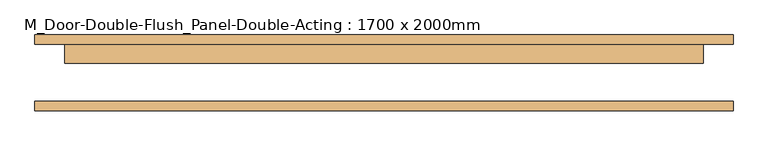
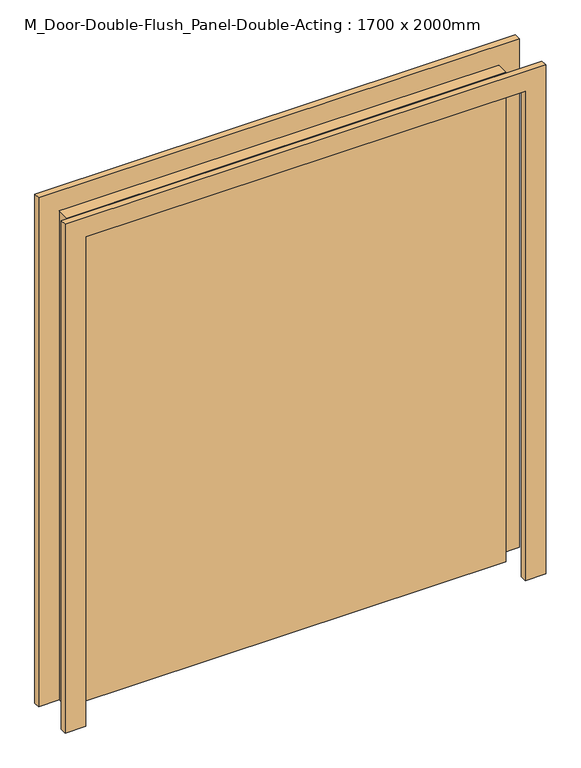
"""IFC4 building model written with IfcOpenShell, lengths in millimetres: door geometry, M_Door-Double-Flush_Panel-Double-Acting : 1700 x 2000mm."""

from ifc_helpers import new_model, si_unit, frame, origin, origin_with_axes, place, context, project, spatial, polyline, outline, extrude, source, transform, mapped, element, save


def m_door_double_flush_panel_double_acting_1700_x_2000mm_82a3dfda(model_context):
    return source(origin(), model_context, "Body", "SweptSolid", [
        extrude(outline(polyline([(2080.0, -930.0), (0.0, -930.0), (0.0, -850.0), (2000.0, -850.0), (2000.0, 850.0), (0.0, 850.0), (0.0, 930.0), (2080.0, 930.0), (2080.0, -930.0)])), frame((0.0, 76.2, 0.0), z_axis=(0.0, 1.0, 0.0), x_axis=(0.0, 0.0, 1.0)), (0.0, 0.0, 1.0), 25.0),
        extrude(outline(polyline([(2000.0, -850.0), (2000.0, 850.0), (0.0, 850.0), (0.0, 930.0), (2080.0, 930.0), (2080.0, -930.0), (0.0, -930.0), (0.0, -850.0), (2000.0, -850.0)])), frame((0.0, -101.2, 0.0), z_axis=(0.0, 1.0, 0.0), x_axis=(0.0, 0.0, 1.0)), (0.0, 0.0, 1.0), 25.0),
        extrude(outline(polyline([(-850.0, 76.2), (850.0, 76.2), (850.0, 26.2), (-850.0, 26.2), (-850.0, 76.2)])), origin_with_axes(), (0.0, 0.0, 1.0), 2000.0),
    ])


if __name__ == "__main__":
    model = new_model("IFC4")
    model_context = context("Model", 3, world=origin())
    ifc_project = project(units=[si_unit("LENGTHUNIT", "METRE", prefix="MILLI")], contexts=[model_context])
    site = spatial("IfcSite", under=ifc_project)
    building = spatial("IfcBuilding", under=site)
    placement = place(None, origin())
    m_door_double_flush_panel_double_acting_1700_x_2000mm_shape = m_door_double_flush_panel_double_acting_1700_x_2000mm_82a3dfda(model_context)
    element("IfcDoor", 1, ObjectType="M_Door-Double-Flush_Panel-Double-Acting : 1700 x 2000mm", at=placement, inside=building, context=model_context, shape_type="MappedRepresentation", body=[
        mapped(m_door_double_flush_panel_double_acting_1700_x_2000mm_shape, transform((0.0, 0.0, 0.0), x_axis=(1.0, 0.0, 0.0), y_axis=(0.0, 1.0, 0.0), z_axis=(0.0, 0.0, 1.0))),
    ])
    save(model, "model.ifc")

# Revit data of these elements
# Type "M_Door-Double-Flush_Panel-Double-Acting : 1700 x 2000mm"
#   Type Mark = "8"
#   Construction Type Id = "DOOR"
#   Assembly Code = "C1020"
#   Analytic Construction = "Wooden"
#   W = 2' - 9.46457"
#   Thickness = 0' - 1.9685"
#   Thermal Resistance (R) = 2.5876 (h·ft²·°F)/BTU
#   Swing Angle [instance default] = 90.00°
#   Heat Transfer Coefficient (U) = 0.3865 BTU/(h·ft²·°F)
#   Height = 6' - 6.74016"
#   Trim Projection Ext. = 0' - 0.98425"
#   Trim Projection Int. = 0' - 0.98425"
#   Trim Width Ext. = 0' - 3.14961"
#   Trim Width Int. = 0' - 3.14961"
#   Width = 5' - 6.92913"
#   Define Thermal Properties by = 1
#   Panel Material = Wood - Birch - Solid Stained Light Low Gloss
#   Trim Material = Paint - Sienna
#   Visual Light Transmittance = 0
#   Solar Heat Gain Coefficient = 0
#   Function = (empty or 0)
#   Wall Closure = (empty or 0)
# Element 1 (IfcDoor, "M_Door-Double-Flush_Panel-Double-Acting : 1700 x 2000mm")
#   Materials on its faces: "Paint - Sienna", "Wood - Birch - Solid Stained Light Low Gloss"
# Materials
#   "Wood - Birch - Solid Stained Light Low Gloss": class "Wood", colour RGB 210 159 95, transparency 0, Cost = 0
#   "Paint - Sienna": colour RGB 118 70 51, transparency 0, Cost = 0
